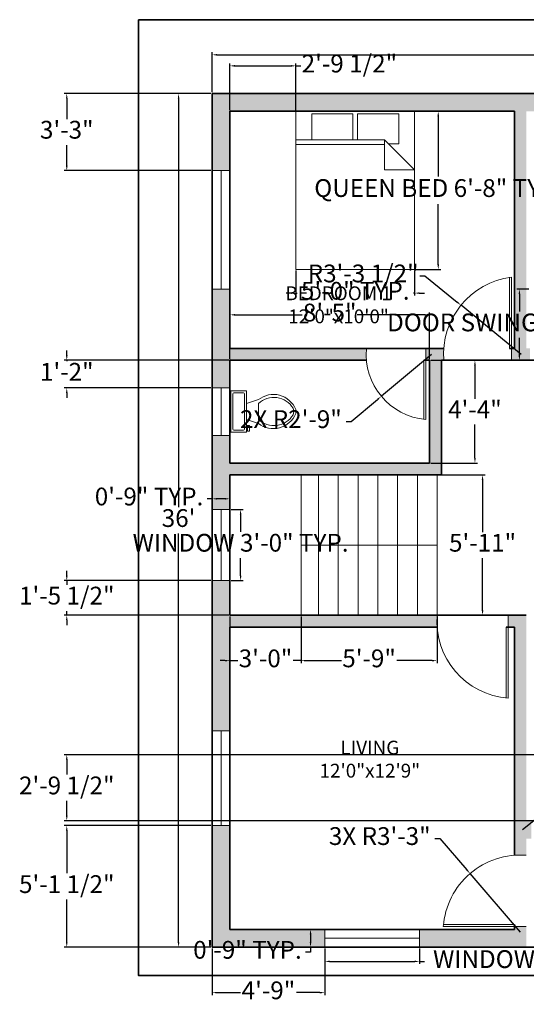
# Model space of a CAD drawing. Units: inches. Extents: x 1649 to 2193, y 1782 to 2280.
# Tile 1 of 3: x 1649 to 1905, y 1782 to 2280. Entities that reach past the tile are written whole.
import ezdxf

# ---------------------------------------------------------------- set-up
doc = ezdxf.new("R2010")
doc.units = ezdxf.units.IN
for name, color, linetype, lineweight in [('A-ANNO-DIMS', 2, 'Continuous', 18), ('A-ANNO-TTLB', 7, 'Continuous', 35), ('A-AREA-IDEN', 7, 'Continuous', 25), ('A-DOOR', 3, 'Continuous', 18), ('A-FLOR-FIXT', 9, 'Continuous', 18), ('A-FLOR-STRS', 7, 'Continuous', 18), ('A-FURN', 8, 'Continuous', 18), ('A-GLAZ', 4, 'Continuous', 18), ('A-WALL', 7, 'Continuous', 35)]:
    doc.layers.add(name, color=color, linetype=linetype, lineweight=lineweight)
doc.layers.add('A-WALL-PATT', color=18, linetype='Continuous', lineweight=13, true_color=0x000000)
doc.styles.get("Standard").update_dxf_attribs({"font": 'arial.ttf'})
doc.dimstyles.new('ISO-25', dxfattribs={"dimtxt": 9, "dimasz": 2.5, "dimexe": 1.25, "dimexo": 0.625, "dimgap": 2, "dimtad": 0, "dimtih": 1, "dimtoh": 1, "dimdec": 1, "dimlunit": 4, "dimtxsty": 'Standard', "dimcen": 2.5, "dimadec": 0, "dimazin": 0, "dimtfac": 0.5, "dimtdec": 1, "dimtmove": 0, "dimatfit": 3, "dimfxl": 1, "dimarcsym": 0})

# ---------------------------------------------------------------- blocks, each defined once
blk = doc.blocks.new('Bed - Queen')
for p, q in [((0, -80.00003), (0, 0)), ((0, 0), (59.99999, 0)), ((59.99999, 0), (59.99999, -80.00003)), ((7.99999, -1.2), (28.79998, -1.2)), ((7.99999, -14.4), (7.99999, -1.2)), ((28.79998, -1.2), (28.79998, -14.4)), ((31.19999, -1.2), (51.99999, -1.2)), ((31.19999, -14.4), (31.19999, -1.2)), ((51.99999, -1.2), (51.99999, -16.4)), ((0, -14.4), (44.8, -14.4)), ((59.99999, -29.6), (44.8, -14.4)), ((44.8, -14.4), (44.8, -29.6)), ((44.8, -16.8), (0, -16.8)), ((51.99999, -16.4), (46.79936, -16.4)), ((44.8, -29.6), (59.99999, -29.6)), ((59.99999, -80.00003), (0, -80.00003))]:
    blk.add_line(p, q)
blk = doc.blocks.new('*U6')
for p, q in [((9.5, -6), (9.5, -2)), ((-10, -8.5), (-8, -8.5)), ((-10, -9.5), (-10, -8.5)), ((-7, -9.5), (-10, -9.5)), ((-8, -8.5), (-8, -8)), ((-7, -8), (-7, -9.5)), ((-4, -8), (-6, -14)), ((4, -8), (6, -14)), ((4, -14), (-4, -14))]:
    blk.add_line(p, q)
blk.add_lwpolyline([(10.5, -8), (10.5, 0), (-10.5, 0), (-10.5, -8)], close=True)
for points in [[(-9.5, -2), (-9.5, -6)], [(8.5, -1), (-8.5, -1)], [(-8.5, -7), (8.5, -7)]]:
    blk.add_lwpolyline(points)
for centre, radius, start, end in [((-8.62, -1.88), 0.884, 81.8699, 188.1301), ((8.62, -1.88), 0.884, 351.8699, 98.1301), ((-8.62, -6.12), 0.884, 171.8699, 278.1301), ((8.62, -6.12), 0.884, 261.8699, 8.1301), ((3.52, -21.58), 12.17, 141.4691, 247.9714), ((4.2, -21.82), 11.33, 136.3677, 238.9468), ((-3.52, -21.58), 12.17, 292.0284, 38.5307), ((-4.2, -21.82), 11.33, 301.053, 43.6321), ((0, -27.88), 4, 245.7318, 294.2682), ((0, -29), 4, 254.8605, 285.1395)]:
    blk.add_arc(centre, radius, start, end)
blk = doc.blocks.new('*D7')
at = {"layer": 'A-ANNO-DIMS', "color": 0, "lineweight": -2, "transparency": 16777216}
for p, q in [((1746.13, 2243.28), (1746.13, 2263.5)), ((1748.63, 2262.25), (1928.49, 2262.25)), ((2127.63, 2262.25), (1947.76, 2262.25)), ((2130.13, 2243.28), (2130.13, 2263.5))]:
    blk.add_line(p, q, dxfattribs=at)
at = {"layer": 'A-ANNO-DIMS', "color": 0, "transparency": 16777216}
for points in [[(1748.63, 2262.67), (1748.63, 2261.83), (1746.13, 2262.25)], [(2127.63, 2262.67), (2127.63, 2261.83), (2130.13, 2262.25)]]:
    blk.add_solid(points, dxfattribs=at)
at = {"layer": 'Defpoints', "color": 0, "transparency": 16777216}
for p in [(2130.13, 2262.25), (1746.13, 2242.65), (2130.13, 2242.65)]:
    blk.add_point(p, dxfattribs=at)
at = {"layer": 'A-ANNO-DIMS', "color": 0, "transparency": 16777216, "insert": (1938.13, 2262.25), "char_height": 9, "attachment_point": 5}
blk.add_mtext("32'", dxfattribs=at)
blk = doc.blocks.new('*D8')
at = {"layer": 'A-ANNO-DIMS', "color": 0, "lineweight": -2, "transparency": 16777216}
for p, q in [((1745.5, 2242.65), (1727.89, 2242.65)), ((1729.14, 2240.15), (1729.14, 2033.25)), ((1729.14, 1813.15), (1729.14, 2020.05)), ((1745.5, 1810.65), (1727.89, 1810.65))]:
    blk.add_line(p, q, dxfattribs=at)
at = {"layer": 'A-ANNO-DIMS', "color": 0, "transparency": 16777216}
for points in [[(1728.72, 2240.15), (1729.55, 2240.15), (1729.14, 2242.65)], [(1728.72, 1813.15), (1729.55, 1813.15), (1729.14, 1810.65)]]:
    blk.add_solid(points, dxfattribs=at)
at = {"layer": 'Defpoints', "color": 0, "transparency": 16777216}
for p in [(1746.13, 2242.65), (1729.14, 1810.65), (1746.13, 1810.65)]:
    blk.add_point(p, dxfattribs=at)
at = {"layer": 'A-ANNO-DIMS', "color": 0, "transparency": 16777216, "insert": (1729.14, 2026.65), "char_height": 9, "attachment_point": 5}
blk.add_mtext("36'", dxfattribs=at)
blk = doc.blocks.new('DOOR-36IN')
for p, q in [((0, 6), (0, 42)), ((1, 6), (1, 42)), ((0, 6), (0, 0))]:
    blk.add_line(p, q)
blk.add_arc((-3, 3), 39.12, 355.6013, 85.6013)
blk = doc.blocks.new('WIN-60IN')
for p, q in [((0, 60), (9, 60)), ((4.5, 60), (4.5, 0)), ((0, 0), (9, 0))]:
    blk.add_line(p, q)
blk = doc.blocks.new('WIN-48IN')
for p, q in [((0, 48), (9, 48)), ((4.5, 48), (4.5, 0)), ((0, 0), (9, 0))]:
    blk.add_line(p, q)
blk = doc.blocks.new('DOOR-30IN')
for p, q in [((0, 6), (0, 36)), ((1, 6), (1, 36)), ((0, 6), (0, 0))]:
    blk.add_line(p, q)
blk.add_arc((-3, 3), 33.14, 354.8056, 84.8056)
blk = doc.blocks.new('WIN-24IN')
for p, q in [((0, 0), (0, 9)), ((24, 0), (24, 9)), ((0, 4.5), (24, 4.5))]:
    blk.add_line(p, q)
blk = doc.blocks.new('WIN-36IN')
for p, q in [((0, 9), (0, 0)), ((36, 9), (36, 0)), ((0, 4.5), (36, 4.5))]:
    blk.add_line(p, q)
blk = doc.blocks.new('*D17')
at = {"layer": 'A-ANNO-DIMS', "color": 0, "lineweight": -2, "transparency": 16777216}
for p, q in [((1906.4, 2143.65), (1900.38, 2143.65)), ((1901.63, 2141.15), (1901.63, 2132.31)), ((1901.63, 2110.15), (1901.63, 2118.99)), ((1906.4, 2107.65), (1900.38, 2107.65))]:
    blk.add_line(p, q, dxfattribs=at)
at = {"layer": 'A-ANNO-DIMS', "color": 0, "transparency": 16777216}
for points in [[(1901.21, 2141.15), (1902.05, 2141.15), (1901.63, 2143.65)], [(1901.21, 2110.15), (1902.05, 2110.15), (1901.63, 2107.65)]]:
    blk.add_solid(points, dxfattribs=at)
at = {"layer": 'Defpoints', "color": 0, "transparency": 16777216}
for p in [(1901.63, 2143.65), (1907.03, 2143.65), (1907.03, 2107.65)]:
    blk.add_point(p, dxfattribs=at)
at = {"layer": 'A-ANNO-DIMS', "color": 0, "transparency": 16777216, "insert": (1901.63, 2125.65), "char_height": 9, "attachment_point": 5}
blk.add_mtext('DOOR SWING 3\'-0" TYP.', dxfattribs=at)
blk = doc.blocks.new('*D21')
at = {"layer": 'A-ANNO-DIMS', "color": 0, "lineweight": -2, "transparency": 16777216}
for p, q in [((1755.75, 2032.15), (1761.78, 2032.15)), ((1760.53, 2029.65), (1760.53, 2020.81)), ((1760.53, 1998.65), (1760.53, 2007.49)), ((1755.75, 1996.15), (1761.78, 1996.15))]:
    blk.add_line(p, q, dxfattribs=at)
at = {"layer": 'A-ANNO-DIMS', "color": 0, "transparency": 16777216}
for points in [[(1760.11, 2029.65), (1760.95, 2029.65), (1760.53, 2032.15)], [(1760.11, 1998.65), (1760.95, 1998.65), (1760.53, 1996.15)]]:
    blk.add_solid(points, dxfattribs=at)
at = {"layer": 'Defpoints', "color": 0, "transparency": 16777216}
for p in [(1755.13, 2032.15), (1760.53, 2032.15), (1755.13, 1996.15)]:
    blk.add_point(p, dxfattribs=at)
at = {"layer": 'A-ANNO-DIMS', "color": 0, "transparency": 16777216, "insert": (1760.53, 2014.15), "char_height": 9, "attachment_point": 5}
blk.add_mtext('WINDOW 3\'-0" TYP.', dxfattribs=at)
blk = doc.blocks.new('*D22')
at = {"layer": 'A-ANNO-DIMS', "color": 0, "lineweight": -2, "transparency": 16777216}
for p, q in [((1746.13, 2032.78), (1746.13, 2038.8)), ((1755.13, 2032.78), (1755.13, 2038.8)), ((1746.13, 2037.55), (1743.63, 2037.55)), ((1752.63, 2037.55), (1748.63, 2037.55))]:
    blk.add_line(p, q, dxfattribs=at)
at = {"layer": 'A-ANNO-DIMS', "color": 0, "transparency": 16777216}
for points in [[(1748.63, 2037.97), (1748.63, 2037.14), (1746.13, 2037.55)], [(1752.63, 2037.97), (1752.63, 2037.14), (1755.13, 2037.55)]]:
    blk.add_solid(points, dxfattribs=at)
at = {"layer": 'Defpoints', "color": 0, "transparency": 16777216}
for p in [(1746.13, 2037.55), (1746.13, 2032.15), (1755.13, 2032.15)]:
    blk.add_point(p, dxfattribs=at)
at = {"layer": 'A-ANNO-DIMS', "color": 0, "transparency": 16777216, "insert": (1714.2, 2037.55), "char_height": 9, "attachment_point": 5}
blk.add_mtext('0\'-9" TYP.', dxfattribs=at)
blk = doc.blocks.new('*D23')
at = {"layer": 'A-ANNO-DIMS', "color": 0, "lineweight": -2, "transparency": 16777216}
for p, q in [((1803.13, 1810.03), (1803.13, 1802.2)), ((1851.13, 1810.03), (1851.13, 1802.2)), ((1805.63, 1803.45), (1848.63, 1803.45)), ((1851.13, 1803.45), (1853.63, 1803.45))]:
    blk.add_line(p, q, dxfattribs=at)
at = {"layer": 'A-ANNO-DIMS', "color": 0, "transparency": 16777216}
for points in [[(1805.63, 1803.87), (1805.63, 1803.04), (1803.13, 1803.45)], [(1848.63, 1803.87), (1848.63, 1803.04), (1851.13, 1803.45)]]:
    blk.add_solid(points, dxfattribs=at)
at = {"layer": 'Defpoints', "color": 0, "transparency": 16777216}
for p in [(1803.13, 1810.65), (1851.13, 1810.65), (1851.13, 1803.45)]:
    blk.add_point(p, dxfattribs=at)
at = {"layer": 'A-ANNO-DIMS', "color": 0, "transparency": 16777216, "insert": (1912.57, 1803.45), "char_height": 9, "attachment_point": 5}
blk.add_mtext('WINDOW 4\'-0" TYP.', dxfattribs=at)
blk = doc.blocks.new('*D24')
at = {"layer": 'A-ANNO-DIMS', "color": 0, "lineweight": -2, "transparency": 16777216}
for p, q in [((1802.5, 1819.65), (1794.68, 1819.65)), ((1795.93, 1817.15), (1795.93, 1813.15)), ((1802.5, 1810.65), (1794.68, 1810.65)), ((1795.93, 1810.65), (1795.93, 1808.15)), ((1795.93, 1808.15), (1793.43, 1808.15))]:
    blk.add_line(p, q, dxfattribs=at)
at = {"layer": 'A-ANNO-DIMS', "color": 0, "transparency": 16777216}
for points in [[(1795.51, 1817.15), (1796.35, 1817.15), (1795.93, 1819.65)], [(1795.51, 1813.15), (1796.35, 1813.15), (1795.93, 1810.65)]]:
    blk.add_solid(points, dxfattribs=at)
at = {"layer": 'Defpoints', "color": 0, "transparency": 16777216}
for p in [(1803.13, 1819.65), (1795.93, 1810.65), (1803.13, 1810.65)]:
    blk.add_point(p, dxfattribs=at)
at = {"layer": 'A-ANNO-DIMS', "color": 0, "transparency": 16777216, "insert": (1764, 1808.15), "char_height": 9, "attachment_point": 5}
blk.add_mtext('0\'-9" TYP.', dxfattribs=at)
blk = doc.blocks.new('*D27')
at = {"layer": 'A-ANNO-DIMS', "color": 0, "lineweight": -2, "transparency": 16777216}
for p, q in [((1849.19, 2233.65), (1861.81, 2233.65)), ((1860.56, 2231.15), (1860.56, 2200.58)), ((1860.56, 2156.15), (1860.56, 2186.72)), ((1849.19, 2153.65), (1861.81, 2153.65))]:
    blk.add_line(p, q, dxfattribs=at)
at = {"layer": 'A-ANNO-DIMS', "color": 0, "transparency": 16777216}
for points in [[(1860.14, 2231.15), (1860.98, 2231.15), (1860.56, 2233.65)], [(1860.14, 2156.15), (1860.98, 2156.15), (1860.56, 2153.65)]]:
    blk.add_solid(points, dxfattribs=at)
at = {"layer": 'Defpoints', "color": 0, "transparency": 16777216}
for p in [(1848.56, 2233.65), (1860.56, 2233.65), (1848.56, 2153.65)]:
    blk.add_point(p, dxfattribs=at)
at = {"layer": 'A-ANNO-DIMS', "color": 0, "transparency": 16777216, "insert": (1860.56, 2193.65), "char_height": 9, "attachment_point": 5}
blk.add_mtext('QUEEN BED 6\'-8" TYP.', dxfattribs=at)
blk = doc.blocks.new('*D28')
at = {"layer": 'A-ANNO-DIMS', "color": 0, "lineweight": -2, "transparency": 16777216}
for p, q in [((1788.56, 2153.03), (1788.56, 2140.4)), ((1848.56, 2153.03), (1848.56, 2140.4)), ((1786.06, 2141.65), (1783.56, 2141.65)), ((1788.56, 2141.65), (1789.13, 2141.65)), ((1848.56, 2141.65), (1847.99, 2141.65)), ((1851.06, 2141.65), (1853.56, 2141.65))]:
    blk.add_line(p, q, dxfattribs=at)
at = {"layer": 'A-ANNO-DIMS', "color": 0, "transparency": 16777216}
for points in [[(1786.06, 2142.07), (1786.06, 2141.24), (1788.56, 2141.65)], [(1851.06, 2142.07), (1851.06, 2141.24), (1848.56, 2141.65)]]:
    blk.add_solid(points, dxfattribs=at)
at = {"layer": 'Defpoints', "color": 0, "transparency": 16777216}
for p in [(1788.56, 2153.65), (1848.56, 2153.65), (1848.56, 2141.65)]:
    blk.add_point(p, dxfattribs=at)
at = {"layer": 'A-ANNO-DIMS', "color": 0, "transparency": 16777216, "insert": (1818.56, 2141.65), "char_height": 9, "attachment_point": 5}
blk.add_mtext('5\'-0" TYP.', dxfattribs=at)
blk = doc.blocks.new('*D33')
at = {"layer": 'A-ANNO-DIMS', "color": 0, "lineweight": -2, "transparency": 16777216}
for p, q in [((1755.13, 2108.28), (1755.13, 2131.9)), ((1757.63, 2130.65), (1791.66, 2130.65)), ((1853.63, 2130.65), (1819.6, 2130.65)), ((1856.13, 2108.28), (1856.13, 2131.9))]:
    blk.add_line(p, q, dxfattribs=at)
at = {"layer": 'A-ANNO-DIMS', "color": 0, "transparency": 16777216}
for points in [[(1757.63, 2131.07), (1757.63, 2130.24), (1755.13, 2130.65)], [(1853.63, 2131.07), (1853.63, 2130.24), (1856.13, 2130.65)]]:
    blk.add_solid(points, dxfattribs=at)
at = {"layer": 'Defpoints', "color": 0, "transparency": 16777216}
for p in [(1856.13, 2130.65), (1755.13, 2107.65), (1856.13, 2107.65)]:
    blk.add_point(p, dxfattribs=at)
at = {"layer": 'A-ANNO-DIMS', "color": 0, "transparency": 16777216, "insert": (1805.63, 2130.65), "char_height": 9, "attachment_point": 5}
blk.add_mtext('8\'-5"', dxfattribs=at)
blk = doc.blocks.new('*D34')
at = {"layer": 'A-ANNO-DIMS', "color": 0, "lineweight": -2, "transparency": 16777216}
for p, q in [((1856.75, 2107.65), (1880.38, 2107.65)), ((1879.13, 2105.15), (1879.13, 2088.15)), ((1879.13, 2058.15), (1879.13, 2075.15)), ((1856.75, 2055.65), (1880.38, 2055.65))]:
    blk.add_line(p, q, dxfattribs=at)
at = {"layer": 'A-ANNO-DIMS', "color": 0, "transparency": 16777216}
for points in [[(1878.71, 2105.15), (1879.55, 2105.15), (1879.13, 2107.65)], [(1878.71, 2058.15), (1879.55, 2058.15), (1879.13, 2055.65)]]:
    blk.add_solid(points, dxfattribs=at)
at = {"layer": 'Defpoints', "color": 0, "transparency": 16777216}
for p in [(1856.13, 2107.65), (1856.13, 2055.65), (1879.13, 2055.65)]:
    blk.add_point(p, dxfattribs=at)
at = {"layer": 'A-ANNO-DIMS', "color": 0, "transparency": 16777216, "insert": (1879.13, 2081.65), "char_height": 9, "attachment_point": 5}
blk.add_mtext('4\'-4"', dxfattribs=at)
blk = doc.blocks.new('*D35')
at = {"layer": 'A-ANNO-DIMS', "color": 0, "lineweight": -2, "transparency": 16777216}
for p, q in [((1860.61, 2049.65), (1884.23, 2049.65)), ((1882.98, 2047.15), (1882.98, 2020.75)), ((1882.98, 1981.15), (1882.98, 2007.56)), ((1860.61, 1978.65), (1884.23, 1978.65))]:
    blk.add_line(p, q, dxfattribs=at)
at = {"layer": 'A-ANNO-DIMS', "color": 0, "transparency": 16777216}
for points in [[(1882.57, 2047.15), (1883.4, 2047.15), (1882.98, 2049.65)], [(1882.57, 1981.15), (1883.4, 1981.15), (1882.98, 1978.65)]]:
    blk.add_solid(points, dxfattribs=at)
at = {"layer": 'Defpoints', "color": 0, "transparency": 16777216}
for p in [(1859.98, 2049.65), (1859.98, 1978.65), (1882.98, 1978.65)]:
    blk.add_point(p, dxfattribs=at)
at = {"layer": 'A-ANNO-DIMS', "color": 0, "transparency": 16777216, "insert": (1882.98, 2014.15), "char_height": 9, "attachment_point": 5}
blk.add_mtext('5\'-11"', dxfattribs=at)
blk = doc.blocks.new('*D38')
at = {"layer": 'A-ANNO-DIMS', "color": 0, "lineweight": -2, "transparency": 16777216}
for p, q in [((1755.13, 1978.03), (1755.13, 1954.4)), ((1791.13, 1978.03), (1791.13, 1954.4)), ((1752.63, 1955.65), (1750.13, 1955.65)), ((1755.13, 1955.65), (1759.17, 1955.65)), ((1791.13, 1955.65), (1787.09, 1955.65)), ((1793.63, 1955.65), (1796.13, 1955.65))]:
    blk.add_line(p, q, dxfattribs=at)
at = {"layer": 'A-ANNO-DIMS', "color": 0, "transparency": 16777216}
for points in [[(1752.63, 1956.07), (1752.63, 1955.24), (1755.13, 1955.65)], [(1793.63, 1956.07), (1793.63, 1955.24), (1791.13, 1955.65)]]:
    blk.add_solid(points, dxfattribs=at)
at = {"layer": 'Defpoints', "color": 0, "transparency": 16777216}
for p in [(1755.13, 1978.65), (1791.13, 1978.65), (1755.13, 1955.65)]:
    blk.add_point(p, dxfattribs=at)
at = {"layer": 'A-ANNO-DIMS', "color": 0, "transparency": 16777216, "insert": (1773.13, 1955.65), "char_height": 9, "attachment_point": 5}
blk.add_mtext('3\'-0"', dxfattribs=at)
blk = doc.blocks.new('*D39')
at = {"layer": 'A-ANNO-DIMS', "color": 0, "lineweight": -2, "transparency": 16777216}
for p, q in [((1791.13, 1978.03), (1791.13, 1954.4)), ((1859.98, 1978.03), (1859.98, 1954.4)), ((1793.63, 1955.65), (1811.59, 1955.65)), ((1857.48, 1955.65), (1839.52, 1955.65))]:
    blk.add_line(p, q, dxfattribs=at)
at = {"layer": 'A-ANNO-DIMS', "color": 0, "transparency": 16777216}
for points in [[(1793.63, 1956.07), (1793.63, 1955.24), (1791.13, 1955.65)], [(1857.48, 1956.07), (1857.48, 1955.24), (1859.98, 1955.65)]]:
    blk.add_solid(points, dxfattribs=at)
at = {"layer": 'Defpoints', "color": 0, "transparency": 16777216}
for p in [(1791.13, 1978.65), (1859.98, 1978.65), (1791.13, 1955.65)]:
    blk.add_point(p, dxfattribs=at)
at = {"layer": 'A-ANNO-DIMS', "color": 0, "transparency": 16777216, "insert": (1825.56, 1955.65), "char_height": 9, "attachment_point": 5}
blk.add_mtext('5\'-9"', dxfattribs=at)
blk = doc.blocks.new('*D40')
at = {"layer": 'A-ANNO-DIMS', "color": 0, "lineweight": -2, "transparency": 16777216}
for p, q in [((1746.13, 1810.03), (1746.13, 1786.4)), ((1803.13, 1810.03), (1803.13, 1786.4)), ((1748.63, 1787.65), (1760.49, 1787.65)), ((1800.63, 1787.65), (1788.77, 1787.65))]:
    blk.add_line(p, q, dxfattribs=at)
at = {"layer": 'A-ANNO-DIMS', "color": 0, "transparency": 16777216}
for points in [[(1748.63, 1788.07), (1748.63, 1787.24), (1746.13, 1787.65)], [(1800.63, 1788.07), (1800.63, 1787.24), (1803.13, 1787.65)]]:
    blk.add_solid(points, dxfattribs=at)
at = {"layer": 'Defpoints', "color": 0, "transparency": 16777216}
for p in [(1746.13, 1810.65), (1803.13, 1810.65), (1803.13, 1787.65)]:
    blk.add_point(p, dxfattribs=at)
at = {"layer": 'A-ANNO-DIMS', "color": 0, "transparency": 16777216, "insert": (1774.63, 1787.65), "char_height": 9, "attachment_point": 5}
blk.add_mtext('4\'-9"', dxfattribs=at)
blk = doc.blocks.new('*D45')
at = {"layer": 'A-ANNO-DIMS', "color": 0, "lineweight": -2, "transparency": 16777216}
for p, q in [((1745.5, 2242.65), (1671.31, 2242.65)), ((1672.56, 2240.15), (1672.56, 2229.75)), ((1672.56, 2206.15), (1672.56, 2216.55)), ((1745.5, 2203.65), (1671.31, 2203.65))]:
    blk.add_line(p, q, dxfattribs=at)
at = {"layer": 'A-ANNO-DIMS', "color": 0, "transparency": 16777216}
for points in [[(1672.15, 2240.15), (1672.98, 2240.15), (1672.56, 2242.65)], [(1672.15, 2206.15), (1672.98, 2206.15), (1672.56, 2203.65)]]:
    blk.add_solid(points, dxfattribs=at)
at = {"layer": 'Defpoints', "color": 0, "transparency": 16777216}
for p in [(1672.56, 2242.65), (1746.13, 2242.65), (1746.13, 2203.65)]:
    blk.add_point(p, dxfattribs=at)
at = {"layer": 'A-ANNO-DIMS', "color": 0, "transparency": 16777216, "insert": (1672.56, 2223.15), "char_height": 9, "attachment_point": 5}
blk.add_mtext('3\'-3"', dxfattribs=at)
blk = doc.blocks.new('*D46')
at = {"layer": 'A-ANNO-DIMS', "color": 0, "lineweight": -2, "transparency": 16777216}
for p, q in [((1672.56, 2110.15), (1672.56, 2112.65)), ((1754.5, 2107.65), (1671.31, 2107.65)), ((1672.56, 2107.65), (1672.56, 2107.17)), ((1745.5, 2093.65), (1671.31, 2093.65)), ((1672.56, 2093.65), (1672.56, 2094.13)), ((1672.56, 2091.15), (1672.56, 2088.65))]:
    blk.add_line(p, q, dxfattribs=at)
at = {"layer": 'A-ANNO-DIMS', "color": 0, "transparency": 16777216}
for points in [[(1672.15, 2110.15), (1672.98, 2110.15), (1672.56, 2107.65)], [(1672.15, 2091.15), (1672.98, 2091.15), (1672.56, 2093.65)]]:
    blk.add_solid(points, dxfattribs=at)
at = {"layer": 'Defpoints', "color": 0, "transparency": 16777216}
for p in [(1672.56, 2107.65), (1755.13, 2107.65), (1746.13, 2093.65)]:
    blk.add_point(p, dxfattribs=at)
at = {"layer": 'A-ANNO-DIMS', "color": 0, "transparency": 16777216, "insert": (1672.56, 2100.65), "char_height": 9, "attachment_point": 5}
blk.add_mtext('1\'-2"', dxfattribs=at)
blk = doc.blocks.new('*D47')
at = {"layer": 'A-ANNO-DIMS', "color": 0, "lineweight": -2, "transparency": 16777216}
for p, q in [((1672.56, 1998.65), (1672.56, 2001.15)), ((1745.5, 1996.15), (1671.31, 1996.15)), ((1672.56, 1996.15), (1672.56, 1994.06)), ((1754.5, 1978.65), (1671.31, 1978.65)), ((1672.56, 1978.65), (1672.56, 1980.75)), ((1672.56, 1976.15), (1672.56, 1973.65))]:
    blk.add_line(p, q, dxfattribs=at)
at = {"layer": 'A-ANNO-DIMS', "color": 0, "transparency": 16777216}
for points in [[(1672.15, 1998.65), (1672.98, 1998.65), (1672.56, 1996.15)], [(1672.15, 1976.15), (1672.98, 1976.15), (1672.56, 1978.65)]]:
    blk.add_solid(points, dxfattribs=at)
at = {"layer": 'Defpoints', "color": 0, "transparency": 16777216}
for p in [(1746.13, 1996.15), (1672.56, 1978.65), (1755.13, 1978.65)]:
    blk.add_point(p, dxfattribs=at)
at = {"layer": 'A-ANNO-DIMS', "color": 0, "transparency": 16777216, "insert": (1672.56, 1987.4), "char_height": 9, "attachment_point": 5}
blk.add_mtext('1\'-5 1/2"', dxfattribs=at)
blk = doc.blocks.new('*D48')
at = {"layer": 'A-ANNO-DIMS', "color": 0, "lineweight": -2, "transparency": 16777216}
for p, q in [((1745.5, 1872.15), (1671.31, 1872.15)), ((1672.56, 1869.65), (1672.56, 1848.06)), ((1672.56, 1813.15), (1672.56, 1834.75)), ((1745.5, 1810.65), (1671.31, 1810.65))]:
    blk.add_line(p, q, dxfattribs=at)
at = {"layer": 'A-ANNO-DIMS', "color": 0, "transparency": 16777216}
for points in [[(1672.15, 1869.65), (1672.98, 1869.65), (1672.56, 1872.15)], [(1672.15, 1813.15), (1672.98, 1813.15), (1672.56, 1810.65)]]:
    blk.add_solid(points, dxfattribs=at)
at = {"layer": 'Defpoints', "color": 0, "transparency": 16777216}
for p in [(1746.13, 1872.15), (1672.56, 1810.65), (1746.13, 1810.65)]:
    blk.add_point(p, dxfattribs=at)
at = {"layer": 'A-ANNO-DIMS', "color": 0, "transparency": 16777216, "insert": (1672.56, 1841.4), "char_height": 9, "attachment_point": 5}
blk.add_mtext('5\'-1 1/2"', dxfattribs=at)
blk = doc.blocks.new('*D52')
at = {"layer": 'A-ANNO-DIMS', "color": 0, "lineweight": -2, "transparency": 16777216}
for p, q in [((1755.13, 2234.28), (1755.13, 2257.9)), ((1788.56, 2234.28), (1788.56, 2257.9)), ((1757.63, 2256.65), (1786.06, 2256.65)), ((1788.56, 2256.65), (1791.06, 2256.65))]:
    blk.add_line(p, q, dxfattribs=at)
at = {"layer": 'A-ANNO-DIMS', "color": 0, "transparency": 16777216}
for points in [[(1757.63, 2257.07), (1757.63, 2256.24), (1755.13, 2256.65)], [(1786.06, 2257.07), (1786.06, 2256.24), (1788.56, 2256.65)]]:
    blk.add_solid(points, dxfattribs=at)
at = {"layer": 'Defpoints', "color": 0, "transparency": 16777216}
for p in [(1788.56, 2256.65), (1755.13, 2233.65), (1788.56, 2233.65)]:
    blk.add_point(p, dxfattribs=at)
at = {"layer": 'A-ANNO-DIMS', "color": 0, "transparency": 16777216, "insert": (1815.59, 2256.65), "char_height": 9, "attachment_point": 5}
blk.add_mtext('2\'-9 1/2"', dxfattribs=at)
blk = doc.blocks.new('*D58')
at = {"layer": 'A-ANNO-DIMS', "color": 0, "lineweight": -2, "transparency": 16777216}
for p, q in [((1994.67, 1908.03), (1671.31, 1908.03)), ((1672.56, 1905.53), (1672.56, 1898)), ((1672.56, 1877.15), (1672.56, 1884.69)), ((1958.5, 1874.65), (1671.31, 1874.65))]:
    blk.add_line(p, q, dxfattribs=at)
at = {"layer": 'A-ANNO-DIMS', "color": 0, "transparency": 16777216}
for points in [[(1672.15, 1905.53), (1672.98, 1905.53), (1672.56, 1908.03)], [(1672.15, 1877.15), (1672.98, 1877.15), (1672.56, 1874.65)]]:
    blk.add_solid(points, dxfattribs=at)
at = {"layer": 'Defpoints', "color": 0, "transparency": 16777216}
for p in [(1995.3, 1908.03), (1672.56, 1874.65), (1959.13, 1874.65)]:
    blk.add_point(p, dxfattribs=at)
at = {"layer": 'A-ANNO-DIMS', "color": 0, "transparency": 16777216, "insert": (1672.56, 1891.34), "char_height": 9, "attachment_point": 5}
blk.add_mtext('2\'-9 1/2"', dxfattribs=at)
blk = doc.blocks.new('*D61')
at = {"layer": 'A-ANNO-DIMS', "color": 0, "lineweight": -2, "transparency": 16777216}
for p, q in [((1954.1, 1910.88), (1936.96, 1897.17)), ((1956.6, 1910.88), (1954.1, 1910.88)), ((1903.19, 1870.15), (1935.01, 1895.61))]:
    blk.add_line(p, q, dxfattribs=at)
at = {"layer": 'A-ANNO-DIMS', "color": 0, "transparency": 16777216}
blk.add_solid([(1936.7, 1897.5), (1937.22, 1896.84), (1935.01, 1895.61)], dxfattribs=at)
at = {"layer": 'Defpoints', "color": 0, "transparency": 16777216}
for p in [(1935.01, 1895.61), (1903.19, 1870.15)]:
    blk.add_point(p, dxfattribs=at)
at = {"layer": 'A-ANNO-DIMS', "color": 0, "transparency": 16777216, "insert": (1985.35, 1910.88), "char_height": 9, "attachment_point": 5}
blk.add_mtext('R3\'-4 1/2"', dxfattribs=at)
blk = doc.blocks.new('*D62')
at = {"layer": 'A-ANNO-DIMS', "color": 0, "lineweight": -2, "transparency": 16777216}
for p, q in [((1851.31, 2150.43), (1853.81, 2150.43)), ((1853.81, 2150.43), (1870.14, 2137.1)), ((1902.52, 2110.65), (1872.08, 2135.51))]:
    blk.add_line(p, q, dxfattribs=at)
at = {"layer": 'A-ANNO-DIMS', "color": 0, "transparency": 16777216}
blk.add_solid([(1870.41, 2137.42), (1869.88, 2136.77), (1872.08, 2135.51)], dxfattribs=at)
at = {"layer": 'Defpoints', "color": 0, "transparency": 16777216}
for p in [(1872.08, 2135.51), (1902.52, 2110.65)]:
    blk.add_point(p, dxfattribs=at)
at = {"layer": 'A-ANNO-DIMS', "color": 0, "transparency": 16777216, "insert": (1822.56, 2150.43), "char_height": 9, "attachment_point": 5}
blk.add_mtext('R3\'-3 1/2"', dxfattribs=at)
blk = doc.blocks.new('*D63')
at = {"layer": 'A-ANNO-DIMS', "color": 0, "lineweight": -2, "transparency": 16777216}
for p, q in [((1858.9, 1865.71), (1861.4, 1865.71)), ((1861.4, 1865.71), (1875.05, 1849.78)), ((1902.13, 1818.19), (1876.67, 1847.89))]:
    blk.add_line(p, q, dxfattribs=at)
at = {"layer": 'A-ANNO-DIMS', "color": 0, "transparency": 16777216}
blk.add_solid([(1875.36, 1850.06), (1874.73, 1849.51), (1876.67, 1847.89)], dxfattribs=at)
at = {"layer": 'Defpoints', "color": 0, "transparency": 16777216}
for p in [(1876.67, 1847.89), (1902.13, 1818.19)]:
    blk.add_point(p, dxfattribs=at)
at = {"layer": 'A-ANNO-DIMS', "color": 0, "transparency": 16777216, "insert": (1830.96, 1865.71), "char_height": 9, "attachment_point": 5}
blk.add_mtext('3X R3\'-3"', dxfattribs=at)
blk = doc.blocks.new('*D64')
at = {"layer": 'A-ANNO-DIMS', "color": 0, "lineweight": -2, "transparency": 16777216}
for p, q in [((1857.23, 2110.65), (1831.77, 2089.44)), ((1816.5, 2076.71), (1829.85, 2087.84)), ((1814, 2076.71), (1816.5, 2076.71))]:
    blk.add_line(p, q, dxfattribs=at)
at = {"layer": 'A-ANNO-DIMS', "color": 0, "transparency": 16777216}
blk.add_solid([(1829.58, 2088.16), (1830.12, 2087.52), (1831.77, 2089.44)], dxfattribs=at)
at = {"layer": 'Defpoints', "color": 0, "transparency": 16777216}
for p in [(1857.23, 2110.65), (1831.77, 2089.44)]:
    blk.add_point(p, dxfattribs=at)
at = {"layer": 'A-ANNO-DIMS', "color": 0, "transparency": 16777216, "insert": (1785.98, 2076.71), "char_height": 9, "attachment_point": 5}
blk.add_mtext('2X R2\'-9"', dxfattribs=at)

msp = doc.modelspace()

# ---------------------------------------------------------------- hatches: boundary and pattern name
at = {"layer": 'A-WALL-PATT'}
h = msp.add_hatch(color=256, dxfattribs=at)
h.dxf.hatch_style = 1
h.paths.add_polyline_path([(1926.13, 2242.65), (1746.13, 2242.65), (1746.13, 2203.65), (1755.13, 2203.65), (1755.13, 2233.65), (1899.13, 2233.65), (1899.13, 2113.65), (1897.63, 2113.65), (1897.63, 2107.65), (1899.13, 2107.65), (1907.03, 2107.65), (1907.03, 2113.65), (1905.13, 2113.65), (1905.13, 2233.65), (1926.13, 2233.65)])
h.paths.add_polyline_path([(2130.13, 2242.65), (1950.13, 2242.65), (1950.13, 2233.65), (1971.13, 2233.65), (1971.13, 2113.65), (1937.03, 2113.65, -0.045361), (1937.03, 2107.65), (1978.81, 2107.65), (1978.81, 2113.65), (1977.13, 2113.65), (1977.13, 2233.65), (2121.13, 2233.65), (2121.13, 2203.65), (2130.13, 2203.65)])
h.paths.add_polyline_path([(2130.13, 2143.65), (2121.13, 2143.65), (2121.13, 2113.65), (2014.81, 2113.65, -0.038405), (2014.81, 2107.65), (2121.13, 2107.65), (2121.13, 2089.15), (2130.13, 2089.15)])
h.paths.add_polyline_path([(1824.23, 2113.65), (1755.13, 2113.65), (1755.13, 2143.65), (1746.13, 2143.65), (1746.13, 2093.65), (1755.13, 2093.65), (1755.13, 2107.65), (1824.23, 2107.65, -0.045361)])
h.paths.add_polyline_path([(1862.13, 2055.65), (1862.13, 2107.65), (1863.33, 2107.65, -0.038218), (1863.33, 2113.65), (1854.23, 2113.65), (1854.23, 2107.65), (1856.13, 2107.65), (1856.13, 2055.65), (1755.13, 2055.65), (1755.13, 2069.65), (1746.13, 2069.65), (1746.13, 2032.15), (1755.13, 2032.15), (1755.13, 2049.65), (1862.13, 2049.65)])
h.paths.add_polyline_path([(2130.13, 2029.15), (2121.13, 2029.15), (2121.13, 2010.65), (2087.48, 2010.65), (2087.48, 2004.65), (2121.13, 2004.65), (2121.13, 1968.65), (2087.48, 1968.65), (2087.48, 1962.65), (2121.13, 1962.65), (2121.13, 1942.65), (2130.13, 1942.65)])
h.paths.add_polyline_path([(2022.13, 1874.65), (1959.13, 1874.65), (1959.13, 1978.65), (1953.13, 1978.65), (1953.13, 1874.65), (1943.69, 1874.65, -0.055385), (1943.69, 1865.65), (2022.13, 1865.65)])
h.paths.add_polyline_path([(2130.13, 1894.65), (2121.13, 1894.65), (2121.13, 1874.65), (2058.13, 1874.65), (2058.13, 1865.65), (2121.13, 1865.65), (2130.13, 1865.65)])
h.paths.add_polyline_path([(1755.13, 1972.65), (1859.98, 1972.65, -0.038405), (1859.98, 1978.65), (1755.13, 1978.65), (1755.13, 1996.15), (1746.13, 1996.15), (1746.13, 1920.15), (1755.13, 1920.15)])
h.paths.add_polyline_path([(1803.13, 1819.65), (1755.13, 1819.65), (1755.13, 1872.15), (1746.13, 1872.15), (1746.13, 1810.65), (1803.13, 1810.65)])
h.paths.add_polyline_path([(1905.13, 1819.65), (1905.13, 1821.19), (1899.13, 1821.19), (1899.13, 1819.65), (1851.13, 1819.65), (1851.13, 1810.65), (1905.13, 1810.65)])
h.paths.add_polyline_path([(1907.69, 1874.65), (1905.13, 1874.65), (1905.13, 1972.65), (1905.13, 1978.65), (1895.98, 1978.65), (1895.98, 1972.65), (1899.13, 1972.65), (1899.13, 1857.19, -0.038405), (1905.13, 1857.19), (1905.13, 1865.65), (1907.69, 1865.65)])

# ---------------------------------------------------------------- linework, layer by layer
at = {"layer": 'A-ANNO-TTLB'}
msp.add_lwpolyline([(1708.93, 2280.02), (2150.99, 2280.02), (2150.99, 1796.25), (1708.93, 1796.25)], close=True, dxfattribs=at)
at = {"layer": 'A-DOOR'}
for p, q in [((1896.63, 2113.65), (1896.63, 2149.65)), ((1897.63, 2113.65), (1897.63, 2149.65)), ((1897.63, 2113.65), (1897.63, 2107.65)), ((1899.13, 1857.19), (1905.13, 1857.19))]:
    msp.add_line(p, q, dxfattribs=at)
msp.add_arc((1902.52, 2110.65), 39.31, 97.1503, 184.3773, dxfattribs=at)
at = {"layer": 'A-FLOR-STRS'}
for p, q in [((1755.13, 2049.65), (1791.13, 2049.65)), ((1791.13, 2049.65), (1791.13, 1978.65)), ((1799.98, 1978.65), (1799.98, 2049.65)), ((1809.98, 1978.65), (1809.98, 2049.65)), ((1819.98, 1978.65), (1819.98, 2049.65)), ((1829.98, 1978.65), (1829.98, 2049.65)), ((1839.98, 1978.65), (1839.98, 2049.65)), ((1849.98, 1978.65), (1849.98, 2049.65)), ((1859.98, 1978.65), (1859.98, 2049.65)), ((1791.13, 2014.15), (1859.98, 2014.15))]:
    msp.add_line(p, q, dxfattribs=at)
at = {"layer": 'A-WALL'}
for p, q in [((1746.13, 2242.65), (2130.13, 2242.65)), ((1746.13, 1810.65), (1746.13, 2242.65)), ((1755.13, 2233.65), (1899.13, 2233.65)), ((1755.13, 2113.65), (1755.13, 2233.65)), ((1899.13, 2113.65), (1899.13, 2233.65)), ((1755.13, 2113.65), (1863.33, 2113.65)), ((1896.63, 2113.65), (1899.13, 2113.65)), ((1755.13, 2107.65), (1824.23, 2107.65)), ((1755.13, 2055.65), (1755.13, 2107.65)), ((1853.23, 2107.65), (1856.13, 2107.65)), ((1856.13, 2055.65), (1856.13, 2107.65)), ((1862.13, 2055.65), (1862.13, 2107.65)), ((1862.13, 2107.65), (1899.13, 2107.65)), ((1899.13, 2107.65), (2121.13, 2107.65)), ((1755.13, 2055.65), (1856.13, 2055.65)), ((1862.13, 2055.65), (1862.13, 2049.65)), ((1755.13, 2049.65), (1862.13, 2049.65)), ((1755.13, 1978.65), (1755.13, 2049.65)), ((1905.13, 1978.65), (1755.13, 1978.65)), ((1755.13, 1819.65), (1755.13, 1972.65)), ((1859.98, 1972.65), (1755.13, 1972.65)), ((1899.13, 1972.65), (1894.98, 1972.65)), ((1899.13, 1857.19), (1899.13, 1972.65)), ((1899.13, 1819.65), (1755.13, 1819.65)), ((1899.13, 1819.65), (1899.13, 1822.19)), ((2130.13, 1810.65), (1746.13, 1810.65))]:
    msp.add_line(p, q, dxfattribs=at)

# ---------------------------------------------------------------- block references
at = {"layer": 'A-DOOR'}
for name, p, rotation in [('DOOR-30IN', (1854.23, 2113.65), 180), ('DOOR-36IN', (1895.98, 1978.65), 180), ('DOOR-36IN', (1905.13, 1821.19), 89.99999999999905)]:
    msp.add_blockref(name, p, dxfattribs=dict(at, rotation=rotation))
at = {"layer": 'A-FLOR-FIXT', "rotation": 89.99999999999999}
msp.add_blockref('*U6', (1755.56, 2081.73), dxfattribs=at)
at = {"layer": 'A-FURN'}
msp.add_blockref('Bed - Queen', (1788.56, 2233.65), dxfattribs=at)
at = {"layer": 'A-GLAZ'}
for name, p, rotation in [('WIN-60IN', (1755.13, 2203.65), 180), ('WIN-24IN', (1755.13, 2069.65), 89.99999999999358), ('WIN-36IN', (1755.13, 1996.15), 89.99999999999916), ('WIN-48IN', (1755.13, 1920.15), 180), ('WIN-48IN', (1803.13, 1819.65), 269.9999999999984)]:
    msp.add_blockref(name, p, dxfattribs=dict(at, rotation=rotation))

# ---------------------------------------------------------------- texts
at = {"layer": 'A-AREA-IDEN', "char_height": 7, "attachment_point": 1}
for s, width, insert in [('\\pxqc;{\\fArial|b1|i0|c0|p34;BEDROOM 1\\P12\'0"x10\'0"}', 84.8314, (1767.69, 2145.06)), ('\\pxqc;{\\fArial|b1|i0|c0|p34;LIVING\\P12\'0"x12\'9"}', 102.5661, (1774.66, 1915.14))]:
    msp.add_mtext_dynamic_manual_height_columns(s, width=width, gutter_width=12.5, heights=[0], dxfattribs=dict(at, insert=insert))

# ---------------------------------------------------------------- dimensions: what is measured, and where the dimension line sits
at = {"layer": 'A-ANNO-DIMS'}
for base, p1, p2, override, picture, middle in [((2130.13, 2262.25), (1746.13, 2242.65), (2130.13, 2242.65), {"dimclrd": 0, "dimclre": 0, "dimclrt": 0}, '*D7', (1938.13, 2262.25)), ((1788.56, 2256.65), (1755.13, 2233.65), (1788.56, 2233.65), {"dimdec": 1, "dimlfac": 1, "dimrnd": 0, "dimzin": 1, "dimdsep": 46, "dimlunit": 4, "dimfrac": 2}, '*D52', (1815.59, 2256.65)), ((1856.13, 2130.65), (1755.13, 2107.65), (1856.13, 2107.65), {"dimdec": 1, "dimlfac": 1, "dimrnd": 0, "dimzin": 1, "dimdsep": 46, "dimlunit": 4, "dimfrac": 2}, '*D33', (1805.63, 2130.65)), ((1803.13, 1787.65), (1746.13, 1810.65), (1803.13, 1810.65), {"dimdec": 1, "dimlfac": 1, "dimrnd": 0, "dimzin": 1, "dimdsep": 46, "dimlunit": 4, "dimfrac": 2}, '*D40', (1774.63, 1787.65))]:
    dim = msp.add_linear_dim(base=base, p1=p1, p2=p2, dimstyle='ISO-25', override=override, dxfattribs=at)
    dim.commit()
    dim.dimension.update_dxf_attribs({"geometry": picture, "text_midpoint": middle})
for base, p1, p2, angle, override, picture, middle in [((1672.56, 2242.65), (1746.13, 2203.65), (1746.13, 2242.65), 90, {"dimdec": 1, "dimlfac": 1, "dimrnd": 0, "dimzin": 1, "dimdsep": 46, "dimlunit": 4, "dimfrac": 2}, '*D45', (1672.56, 2223.15)), ((1729.14, 1810.65), (1746.13, 2242.65), (1746.13, 1810.65), 90, {"dimclrd": 0, "dimclre": 0, "dimclrt": 0}, '*D8', (1729.14, 2026.65)), ((1672.56, 2107.65), (1746.13, 2093.65), (1755.13, 2107.65), 90, {"dimdec": 1, "dimlfac": 1, "dimrnd": 0, "dimzin": 1, "dimdsep": 46, "dimlunit": 4, "dimfrac": 2}, '*D46', (1672.56, 2100.65)), ((1879.13, 2055.65), (1856.13, 2107.65), (1856.13, 2055.65), 270, {"dimdec": 1, "dimlfac": 1, "dimrnd": 0, "dimzin": 1, "dimdsep": 46, "dimlunit": 4, "dimfrac": 2}, '*D34', (1879.13, 2081.65)), ((1882.98, 1978.65), (1859.98, 2049.65), (1859.98, 1978.65), 270, {"dimdec": 1, "dimlfac": 1, "dimrnd": 0, "dimzin": 1, "dimdsep": 46, "dimlunit": 4, "dimfrac": 2}, '*D35', (1882.98, 2014.15)), ((1672.56, 1978.65), (1746.13, 1996.15), (1755.13, 1978.65), 90, {"dimdec": 1, "dimlfac": 1, "dimrnd": 0, "dimzin": 1, "dimdsep": 46, "dimlunit": 4, "dimfrac": 2}, '*D47', (1672.56, 1987.4)), ((1755.13, 1955.65), (1791.13, 1978.65), (1755.13, 1978.65), 180, {"dimdec": 1, "dimlfac": 1, "dimrnd": 0, "dimzin": 1, "dimdsep": 46, "dimlunit": 4, "dimfrac": 2}, '*D38', (1773.13, 1955.65)), ((1791.1289, 1955.6524), (1859.9831, 1978.6524), (1791.1289, 1978.6524), 180, {"dimdec": 1, "dimlfac": 1, "dimrnd": 0, "dimzin": 1, "dimdsep": 46, "dimlunit": 4, "dimfrac": 2}, '*D39', (1825.556, 1955.6524)), ((1672.56, 1874.65), (1995.3, 1908.03), (1959.13, 1874.65), 90, {"dimdec": 1, "dimlfac": 1, "dimrnd": 0, "dimzin": 1, "dimdsep": 46, "dimlunit": 4, "dimfrac": 2}, '*D58', (1672.56, 1891.34)), ((1672.56, 1810.65), (1746.13, 1872.15), (1746.13, 1810.65), 90, {"dimdec": 1, "dimlfac": 1, "dimrnd": 0, "dimzin": 1, "dimdsep": 46, "dimlunit": 4, "dimfrac": 2}, '*D48', (1672.56, 1841.4))]:
    dim = msp.add_linear_dim(base=base, p1=p1, p2=p2, angle=angle, dimstyle='ISO-25', override=override, dxfattribs=at)
    dim.commit()
    dim.dimension.update_dxf_attribs({"geometry": picture, "text_midpoint": middle})
for base, p1, p2, angle, text, picture, middle in [((1860.56, 2233.65), (1848.56, 2153.65), (1848.56, 2233.65), 90, 'QUEEN BED <> TYP.', '*D27', (1860.56, 2193.65)), ((1901.63, 2143.65), (1907.03, 2107.65), (1907.03, 2143.65), 90, 'DOOR SWING <> TYP.', '*D17', (1901.63, 2125.65)), ((1746.13, 2037.55), (1755.13, 2032.15), (1746.13, 2032.15), 180, '<> TYP.', '*D22', (1714.2, 2037.55)), ((1760.53, 2032.15), (1755.13, 1996.15), (1755.13, 2032.15), 90, 'WINDOW <> TYP.', '*D21', (1760.53, 2014.15)), ((1795.93, 1810.65), (1803.13, 1819.65), (1803.13, 1810.65), 270, '<> TYP.', '*D24', (1764, 1808.15))]:
    dim = msp.add_linear_dim(base=base, p1=p1, p2=p2, angle=angle, text=text, dimstyle='ISO-25', override={"dimdec": 1, "dimlfac": 1, "dimrnd": 0, "dimzin": 1, "dimdsep": 46, "dimlunit": 4, "dimfrac": 2}, dxfattribs=at)
    dim.commit()
    dim.dimension.update_dxf_attribs({"geometry": picture, "text_midpoint": middle})
for center, mpoint, picture, middle in [((1902.52, 2110.65), (1872.08, 2135.51), '*D62', (1822.56, 2150.43)), ((1903.1856, 1870.1524), (1935.0054, 1895.6083), '*D61', (1985.3516, 1910.8818))]:
    dim = msp.add_radius_dim(center=center, mpoint=mpoint, dimstyle='ISO-25', override={"dimdec": 1, "dimlfac": 1, "dimrnd": 0, "dimzin": 1, "dimdsep": 46, "dimlunit": 4, "dimfrac": 2}, dxfattribs=at)
    dim.commit()
    dim.dimension.update_dxf_attribs({"geometry": picture, "text_midpoint": middle, "dimtype": 164})
for base, p1, p2, text, picture, middle in [((1848.56, 2141.65), (1788.56, 2153.65), (1848.56, 2153.65), '<> TYP.', '*D28', (1818.56, 2141.65)), ((1851.13, 1803.45), (1803.13, 1810.65), (1851.13, 1810.65), 'WINDOW <> TYP.', '*D23', (1912.57, 1803.45))]:
    dim = msp.add_linear_dim(base=base, p1=p1, p2=p2, text=text, dimstyle='ISO-25', override={"dimdec": 1, "dimlfac": 1, "dimrnd": 0, "dimzin": 1, "dimdsep": 46, "dimlunit": 4, "dimfrac": 2}, dxfattribs=at)
    dim.commit()
    dim.dimension.update_dxf_attribs({"geometry": picture, "text_midpoint": middle})
for center, mpoint, text, picture, middle in [((1857.23, 2110.65), (1831.77, 2089.44), '2X <>', '*D64', (1785.98, 2076.71)), ((1902.13, 1818.19), (1876.67, 1847.89), '3X <>', '*D63', (1830.96, 1865.71))]:
    dim = msp.add_radius_dim(center=center, mpoint=mpoint, text=text, dimstyle='ISO-25', override={"dimdec": 1, "dimlfac": 1, "dimrnd": 0, "dimzin": 1, "dimdsep": 46, "dimlunit": 4, "dimfrac": 2}, dxfattribs=at)
    dim.commit()
    dim.dimension.update_dxf_attribs({"geometry": picture, "text_midpoint": middle, "dimtype": 164})

doc.saveas('drawing.dxf')
